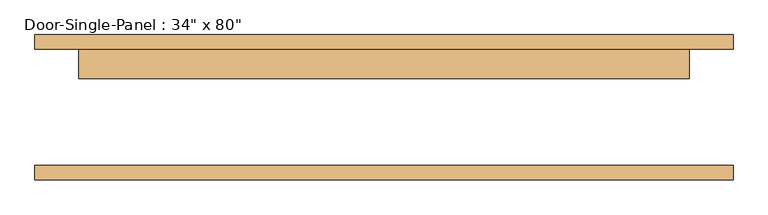
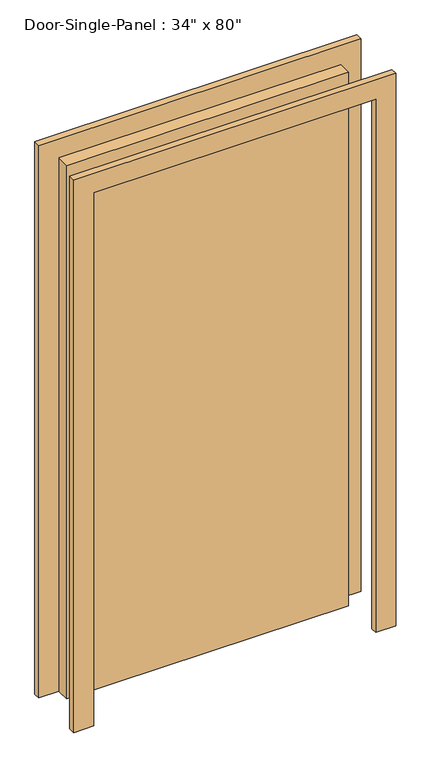
"""IFC4 building model written with IfcOpenShell, lengths in millimetres: door geometry."""

from ifc_helpers import new_model, si_unit, frame, origin, origin_with_axes, place, context, project, spatial, polyline, outline, extrude, source, transform, mapped, element, save


def door_ed2803e5(model_context):
    return source(origin(), model_context, "Body", "SweptSolid", [
        extrude(outline(polyline([(533.4, 50.8), (-533.4, 50.8), (-533.4, 101.6), (533.4, 101.6), (533.4, 50.8)])), origin_with_axes(), (0.0, 0.0, 1.0), 2133.6),
        extrude(outline(polyline([(2209.8, -609.6), (0.0, -609.6), (0.0, -533.4), (2133.6, -533.4), (2133.6, 533.4), (0.0, 533.4), (0.0, 609.6), (2209.8, 609.6), (2209.8, -609.6)])), frame((0.0, 101.6, 0.0), z_axis=(0.0, 1.0, 0.0), x_axis=(0.0, 0.0, 1.0)), (0.0, 0.0, 1.0), 25.4),
        extrude(outline(polyline([(2209.8, 609.6), (2209.8, -609.6), (0.0, -609.6), (0.0, -533.4), (2133.6, -533.4), (2133.6, 533.4), (0.0, 533.4), (0.0, 609.6), (2209.8, 609.6)])), frame((0.0, -127.0, 0.0), z_axis=(0.0, 1.0, 0.0), x_axis=(0.0, 0.0, 1.0)), (0.0, 0.0, 1.0), 25.4),
    ])


if __name__ == "__main__":
    model = new_model("IFC4")
    model_context = context("Model", 3, world=origin())
    ifc_project = project(units=[si_unit("LENGTHUNIT", "METRE", prefix="MILLI")], contexts=[model_context])
    site = spatial("IfcSite", under=ifc_project)
    building = spatial("IfcBuilding", under=site)
    placement = place(None, origin())
    door_shape = door_ed2803e5(model_context)
    element("IfcDoor", 1, ObjectType="Door-Single-Panel : 34\" x 80\"", at=placement, inside=building, context=model_context, shape_type="MappedRepresentation", body=[
        mapped(door_shape, transform((0.0, 0.0, 0.0), x_axis=(1.0, 0.0, 0.0), y_axis=(0.0, 1.0, 0.0), z_axis=(0.0, 0.0, 1.0))),
    ])
    save(model, "model.ifc")

# Revit data of these elements
# Type "Door-Single-Panel : 34\" x 80\""
#   Type Mark = "8"
#   Construction Type Id = "DOOR"
#   Assembly Code = "C1020300"
#   Analytic Construction = "Wooden"
#   Thickness = 0' - 2"
#   Thermal Resistance (R) = 2.5876 (h·ft²·°F)/BTU
#   Swing Angle [instance default] = 90.00°
#   Heat Transfer Coefficient (U) = 0.3865 BTU/(h·ft²·°F)
#   Height = 7' - 0"
#   Trim Projection Ext = 0' - 1"
#   Trim Projection Int = 0' - 1"
#   Trim Width = 0' - 3"
#   Width = 3' - 6"
#   Define Thermal Properties by = 1
#   Panel Material = Wood - Birch - Solid Stained Light Low Gloss
#   Trim Material = Paint - Sienna
#   Visual Light Transmittance = 0
#   Solar Heat Gain Coefficient = 0
#   Function = (empty or 0)
#   Wall Closure = (empty or 0)
# Element 1 (IfcDoor, "Door-Single-Panel : 34\" x 80\"")
#   Materials on its faces: "Paint - Sienna", "Wood - Birch - Solid Stained Light Low Gloss"
# Materials
#   "Wood - Birch - Solid Stained Light Low Gloss": class "Wood", colour RGB 210 159 95, transparency 0, Cost = 0
#   "Paint - Sienna": colour RGB 118 70 51, transparency 0, Cost = 0
